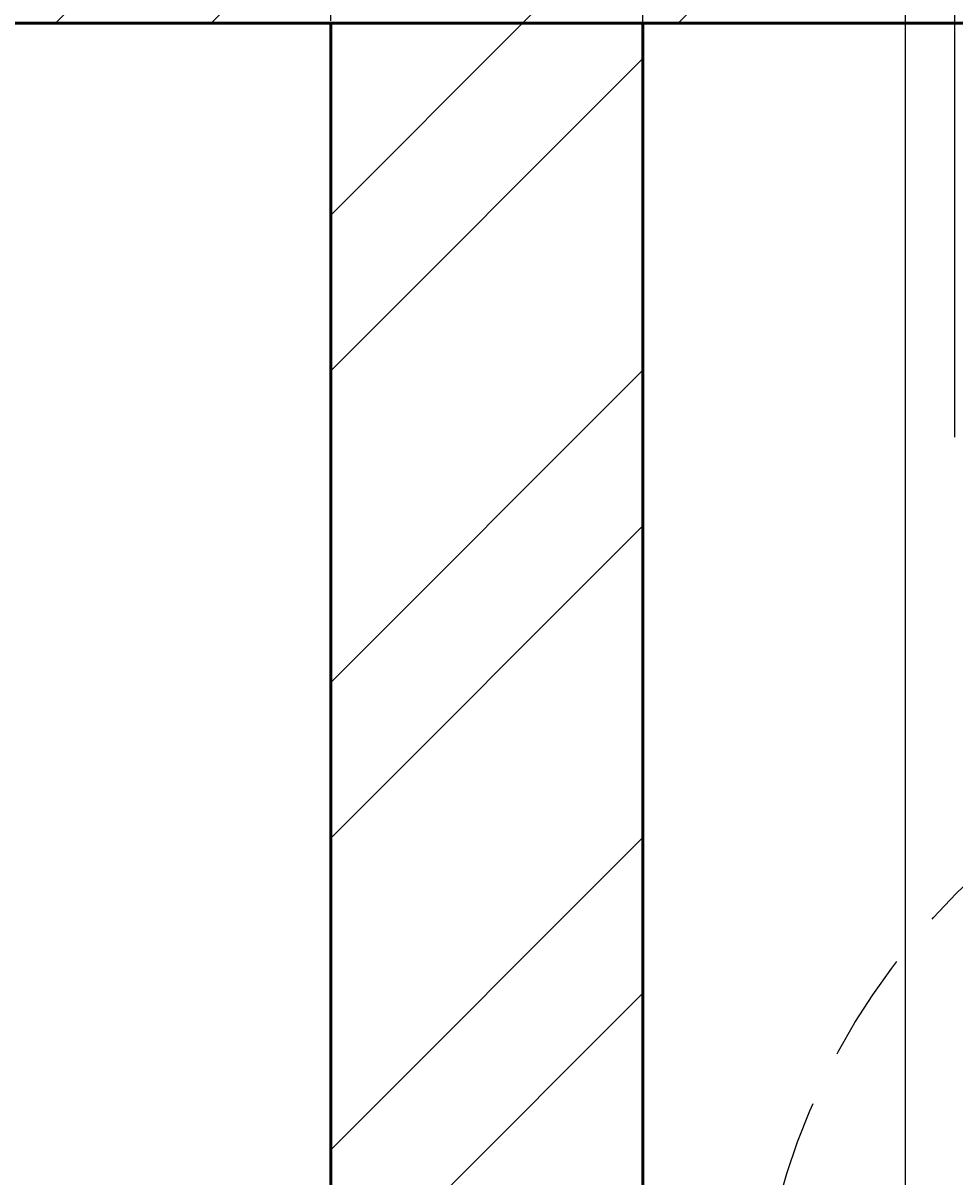
# Model space of a CAD drawing. Units: inches. Extents: x 2812 to 3051, y 1398 to 1659.
# Tile 62 of 65: x 2944 to 2970, y 1605 to 1638. Entities that reach past the tile are written whole.
import ezdxf

# ---------------------------------------------------------------- set-up
doc = ezdxf.new("R2010")
doc.units = ezdxf.units.IN
doc.linetypes.add('HIDDEN2', pattern=[4.7625, 3.175, -1.5875])
for name, color, linetype, lineweight in [('A-ANNO-DIMS', 2, 'Continuous', 18), ('S-CONC', 7, 'Continuous', 50), ('S-CONC-HIDN', 8, 'HIDDEN2', 25), ('S-CONC-PATT', 8, 'Continuous', 18)]:
    doc.layers.add(name, color=color, linetype=linetype, lineweight=lineweight)
doc.styles.get("Standard").update_dxf_attribs({"font": 'arial.ttf'})
doc.dimstyles.get("Standard").update_dxf_attribs({"dimtxt": 0.18, "dimasz": 0.18, "dimexe": 0.18, "dimexo": 0.0625, "dimgap": 0.09, "dimtad": 0, "dimtih": 1, "dimtoh": 1, "dimdec": 4, "dimzin": 0, "dimdsep": 46, "dimtxsty": 'Standard', "dimcen": 0.09, "dimadec": 0, "dimazin": 0, "dimtfac": 1, "dimtdec": 4, "dimtofl": 0, "dimtmove": 0, "dimatfit": 3, "dimfxl": 1, "dimtolj": 1, "dimtzin": 0, "dimarcsym": 0})

# ---------------------------------------------------------------- blocks, each defined once
blk = doc.blocks.new('*D20')
at = {"layer": 'A-ANNO-DIMS', "color": 0, "lineweight": -2, "transparency": 16777216}
for p, q in [((2941.385, 1625.882), (2941.385, 1659.35)), ((2952.385, 1637.882), (2952.385, 1659.35)), ((2941.565, 1659.17), (2946.692, 1659.17)), ((2952.205, 1659.17), (2947.078, 1659.17))]:
    blk.add_line(p, q, dxfattribs=at)
at = {"layer": 'A-ANNO-DIMS', "color": 0, "transparency": 16777216}
for points in [[(2941.565, 1659.2), (2941.565, 1659.14), (2941.385, 1659.17)], [(2952.205, 1659.2), (2952.205, 1659.14), (2952.385, 1659.17)]]:
    blk.add_solid(points, dxfattribs=at)
at = {"layer": 'Defpoints', "color": 0, "transparency": 16777216}
for p in [(2952.385, 1659.17), (2952.385, 1637.82), (2941.385, 1625.82)]:
    blk.add_point(p, dxfattribs=at)
at = {"layer": 'A-ANNO-DIMS', "color": 0, "transparency": 16777216, "insert": (2946.885, 1659.17), "char_height": 0.18, "attachment_point": 5}
blk.add_mtext('\\A1;11', dxfattribs=at)
blk = doc.blocks.new('*D22')
at = {"layer": 'A-ANNO-DIMS', "color": 0, "lineweight": -2, "transparency": 16777216}
for p, q in [((2961.385, 1637.882), (2961.385, 1659.35)), ((2970.385, 1625.882), (2970.385, 1659.35)), ((2961.565, 1659.17), (2965.736, 1659.17)), ((2970.205, 1659.17), (2966.034, 1659.17))]:
    blk.add_line(p, q, dxfattribs=at)
at = {"layer": 'A-ANNO-DIMS', "color": 0, "transparency": 16777216}
for points in [[(2961.565, 1659.2), (2961.565, 1659.14), (2961.385, 1659.17)], [(2970.205, 1659.2), (2970.205, 1659.14), (2970.385, 1659.17)]]:
    blk.add_solid(points, dxfattribs=at)
at = {"layer": 'Defpoints', "color": 0, "transparency": 16777216}
for p in [(2970.385, 1659.17), (2961.385, 1637.82), (2970.385, 1625.82)]:
    blk.add_point(p, dxfattribs=at)
at = {"layer": 'A-ANNO-DIMS', "color": 0, "transparency": 16777216, "insert": (2965.885, 1659.17), "char_height": 0.18, "attachment_point": 5}
blk.add_mtext('\\A1;9', dxfattribs=at)
blk = doc.blocks.new('*D23')
at = {"layer": 'A-ANNO-DIMS', "color": 0, "lineweight": -2, "transparency": 16777216}
for p, q in [((2970.385, 1625.882), (2970.385, 1659.35)), ((2979.385, 1625.882), (2979.385, 1659.35)), ((2970.565, 1659.17), (2974.736, 1659.17)), ((2979.205, 1659.17), (2975.034, 1659.17))]:
    blk.add_line(p, q, dxfattribs=at)
at = {"layer": 'A-ANNO-DIMS', "color": 0, "transparency": 16777216}
for points in [[(2970.565, 1659.2), (2970.565, 1659.14), (2970.385, 1659.17)], [(2979.205, 1659.2), (2979.205, 1659.14), (2979.385, 1659.17)]]:
    blk.add_solid(points, dxfattribs=at)
at = {"layer": 'Defpoints', "color": 0, "transparency": 16777216}
for p in [(2979.385, 1659.17), (2970.385, 1625.82), (2979.385, 1625.82)]:
    blk.add_point(p, dxfattribs=at)
at = {"layer": 'A-ANNO-DIMS', "color": 0, "transparency": 16777216, "insert": (2974.885, 1659.17), "char_height": 0.18, "attachment_point": 5}
blk.add_mtext('\\A1;9', dxfattribs=at)
blk = doc.blocks.new('*D69')
at = {"layer": 'A-ANNO-DIMS', "color": 0, "lineweight": -2, "transparency": 16777216}
for p, q in [((2961.385, 1472.098), (2961.385, 1659.35)), ((2968.956, 1467.81), (2968.956, 1659.35)), ((2961.565, 1659.17), (2964.795, 1659.17)), ((2968.776, 1659.17), (2965.546, 1659.17))]:
    blk.add_line(p, q, dxfattribs=at)
at = {"layer": 'A-ANNO-DIMS', "color": 0, "transparency": 16777216}
for points in [[(2961.565, 1659.2), (2961.565, 1659.14), (2961.385, 1659.17)], [(2968.776, 1659.2), (2968.776, 1659.14), (2968.956, 1659.17)]]:
    blk.add_solid(points, dxfattribs=at)
at = {"layer": 'Defpoints', "color": 0, "transparency": 16777216}
for p in [(2968.956, 1659.17), (2961.385, 1472.035), (2968.956, 1467.747)]:
    blk.add_point(p, dxfattribs=at)
at = {"layer": 'A-ANNO-DIMS', "color": 0, "transparency": 16777216, "insert": (2965.17, 1659.17), "char_height": 0.18, "attachment_point": 5}
blk.add_mtext('\\A1;7.571', dxfattribs=at)

msp = doc.modelspace()

# ---------------------------------------------------------------- hatches: boundary and pattern name
at = {"layer": 'S-CONC-PATT'}
h = msp.add_hatch(dxfattribs=at)
h.set_pattern_fill('ANSI32', color=256)
h.paths.add_polyline_path([(3027.3849, 1646.82), (2835.3849, 1646.82), (2835.3849, 1603.2296), (2844.3849, 1603.2296), (2844.3849, 1637.82), (3018.3849, 1637.82), (3018.3849, 1602.5441), (3027.3849, 1602.5441)])
h.paths.add_polyline_path([(2844.3849, 1594.2296), (2835.3849, 1594.2296), (2835.3849, 1550.82), (3027.3849, 1550.82), (3027.3849, 1593.5441), (3018.3849, 1593.5441), (3018.3849, 1559.82), (2844.3849, 1559.82)])
h.paths.add_polyline_path([(2844.3849, 1482.0354), (2835.3849, 1482.0354), (2835.3849, 1463.4959), (2844.3849, 1463.4959)])
h.paths.add_polyline_path([(2844.3849, 1461.4959), (2835.3849, 1461.4959), (2835.3849, 1416.0354), (2844.3849, 1416.0354)])
h.paths.add_polyline_path([(3027.3849, 1482.0354), (3018.3849, 1482.0354), (3018.3849, 1463.2854), (3027.3849, 1463.2854)])
h.paths.add_polyline_path([(3027.3849, 1461.2854), (3018.3849, 1461.2854), (3018.3849, 1416.0354), (3027.3849, 1416.0354)])
h.paths.add_polyline_path([(2961.3849, 1448.4738), (2952.3849, 1448.4738), (2952.3849, 1416.0354), (2961.3849, 1416.0354)])
h.paths.add_polyline_path([(2961.3849, 1462.3026), (2952.3849, 1462.3026), (2952.3849, 1450.4738), (2961.3849, 1450.4738)])
h.paths.add_polyline_path([(2961.3849, 1472.0354), (2952.3849, 1472.0354), (2952.3849, 1462.3026), (2961.3849, 1462.3026)])
h = msp.add_hatch(dxfattribs=at)
h.set_pattern_fill('ANSI32', color=256)
h.paths.add_polyline_path([(2961.3849, 1637.82), (2952.3849, 1637.82), (2952.3849, 1603.2541), (2961.3849, 1603.2541)])
h.paths.add_polyline_path([(2961.3849, 1594.2541), (2952.3849, 1594.2541), (2952.3849, 1559.82), (2961.3849, 1559.82)])
h.paths.add_polyline_path([(2883.3849, 1637.82), (2880.3849, 1637.82), (2880.3849, 1559.82), (2883.3849, 1559.82)])

# ---------------------------------------------------------------- linework, layer by layer
at = {"layer": 'S-CONC'}
for p, q in [((2844.3849, 1637.82), (3018.3849, 1637.82)), ((2952.3849, 1637.82), (2952.3849, 1559.82)), ((2961.3849, 1559.82), (2961.3849, 1637.82))]:
    msp.add_line(p, q, dxfattribs=at)
at = {"layer": 'S-CONC-HIDN'}
msp.add_circle((2984.3156, 1598.82), 19.6588, dxfattribs=at)

# ---------------------------------------------------------------- dimensions: what is measured, and where the dimension line sits
at = {"layer": 'A-ANNO-DIMS'}
for base, p1, p2, override, picture, middle in [((2952.3849, 1659.17), (2941.3849, 1625.82), (2952.3849, 1637.82), {"dimdec": 0, "dimlfac": 1, "dimrnd": 0, "dimzin": 0, "dimdsep": 46, "dimlunit": 2}, '*D20', (2946.8849, 1659.17)), ((2970.3849, 1659.17), (2961.3849, 1637.82), (2970.3849, 1625.82), {"dimdec": 0, "dimlfac": 1, "dimrnd": 0, "dimzin": 0, "dimdsep": 46, "dimlunit": 2}, '*D22', (2965.8849, 1659.17)), ((2968.9558, 1659.17), (2961.3849, 1472.0354), (2968.9558, 1467.7474), {"dimdec": 3, "dimlfac": 1, "dimrnd": 0, "dimzin": 0, "dimdsep": 46, "dimlunit": 2}, '*D69', (2965.1704, 1659.17)), ((2979.3849, 1659.17), (2970.3849, 1625.82), (2979.3849, 1625.82), {"dimdec": 0, "dimlfac": 1, "dimrnd": 0, "dimzin": 0, "dimdsep": 46, "dimlunit": 2}, '*D23', (2974.8849, 1659.17))]:
    dim = msp.add_linear_dim(base=base, p1=p1, p2=p2, dimstyle='Standard', override=override, dxfattribs=at)
    dim.commit()
    dim.dimension.update_dxf_attribs({"geometry": picture, "text_midpoint": middle})

doc.saveas('drawing.dxf')
